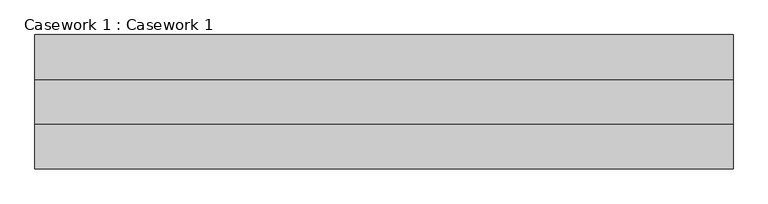
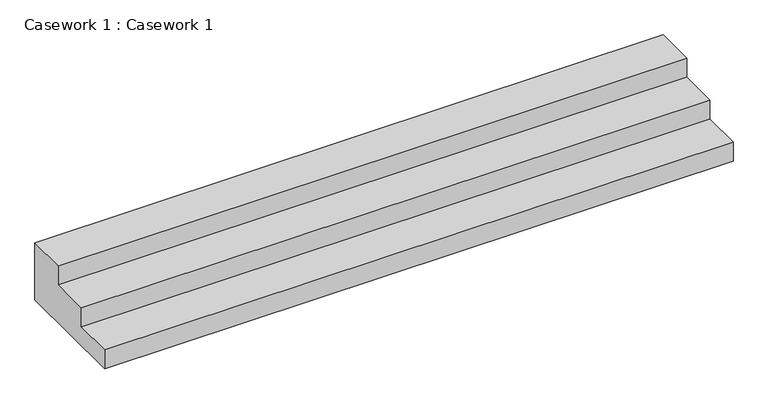
"""IFC4 building model written with IfcOpenShell, lengths in millimetres: furniture geometry, Casework 1 : Casework 1."""

from ifc_helpers import new_model, si_unit, frame, origin, place, context, project, spatial, polyline, outline, extrude, source, transform, mapped, element, save


def casework_1_casework_1_eb7a94e5(model_context):
    return source(origin(), model_context, "Body", "SweptSolid", [
        extrude(outline(polyline([(-1367.7436924, 457.2), (-1062.9436924, 457.2), (-1062.9436924, 0.0), (-1977.3436924, 0.0), (-1977.3436924, 152.4), (-1672.5436924, 152.4), (-1672.5436924, 304.8), (-1367.7436924, 304.8), (-1367.7436924, 457.2)])), frame((-2301.2726479, 0.0, 0.0), z_axis=(1.0, 0.0, 0.0), x_axis=(0.0, 1.0, 0.0)), (0.0, 0.0, 1.0), 4757.3227882),
    ])


if __name__ == "__main__":
    model = new_model("IFC4")
    model_context = context("Model", 3, world=origin())
    ifc_project = project(units=[si_unit("LENGTHUNIT", "METRE", prefix="MILLI")], contexts=[model_context])
    site = spatial("IfcSite", under=ifc_project)
    building = spatial("IfcBuilding", under=site)
    placement = place(None, origin())
    casework_1_casework_1_shape = casework_1_casework_1_eb7a94e5(model_context)
    element("IfcFurniture", 1, ObjectType="Casework 1 : Casework 1", at=placement, inside=building, context=model_context, shape_type="MappedRepresentation", body=[
        mapped(casework_1_casework_1_shape, transform((0.0, 0.0, 0.0), x_axis=(1.0, 0.0, 0.0), y_axis=(0.0, 1.0, 0.0), z_axis=(0.0, 0.0, 1.0))),
    ])
    save(model, "model.ifc")

# Revit data of these elements
# Element 1 (IfcFurniture, "Casework 1 : Casework 1")
#   Materials on its faces: "Asphalt Shingle"
# Materials
#   "Asphalt Shingle": class "Generic", colour RGB 155 155 155, transparency 0, Description = "Asphalt roofing shingle", Cost = 0
